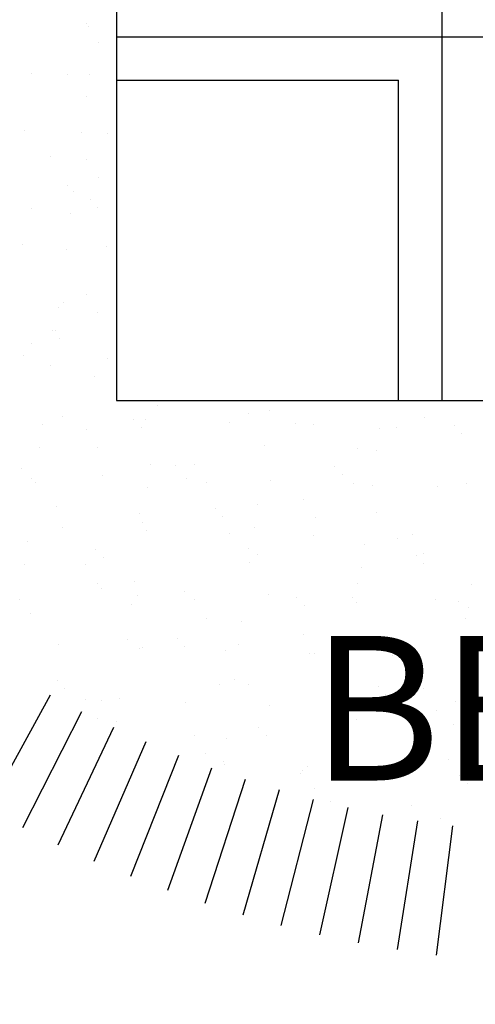
# Model space of a CAD drawing. Units: millimetres. Extents: x -857 to 54106, y -13666 to 13947.
# Tile 32 of 41: x 31622 to 32096, y 8428 to 9453. Entities that reach past the tile are written whole.
import ezdxf

# ---------------------------------------------------------------- set-up
doc = ezdxf.new("R2010")
doc.units = ezdxf.units.MM
for name, color, linetype, lineweight in [('A-ANNO-DIMS', 2, 'Continuous', 18), ('A-AREA-IDEN', 3, 'Continuous', 18), ('A-FURN', 21, 'Continuous', 18)]:
    doc.layers.add(name, color=color, linetype=linetype, lineweight=lineweight)
for name, color, linetype in [('A-FRN', 11, 'Continuous'), ('A-HT', 15, 'Continuous'), ('L-HT', 1, 'Continuous')]:
    doc.layers.add(name, color=color, linetype=linetype)
doc.styles.get("Standard").update_dxf_attribs({"font": 'arial.ttf'})
doc.dimstyles.new('ISO-25', dxfattribs={"dimtxt": 2.5, "dimasz": 2.5, "dimexe": 1.25, "dimexo": 0.625, "dimtad": 1, "dimtxsty": 'Standard', "dimcen": 2.5, "dimadec": 0, "dimazin": 0, "dimtfac": 1, "dimtmove": 0, "dimatfit": 3, "dimfxl": 1, "dimarcsym": 0})

# ---------------------------------------------------------------- blocks, each defined once
blk = doc.blocks.new('*X18')
at = {"color": 0}
for p, q in [((3.0291, 2.2112), (3.0291, 2.2112)), ((2.489, 2.2062), (2.489, 2.2062)), ((2.6199, 2.2078), (2.6199, 2.2078)), ((2.7478, 2.2072), (2.7478, 2.2072)), ((2.8787, 2.2094), (2.8787, 2.2094)), ((2.9625, 2.2024), (2.9625, 2.2024)), ((2.9885, 2.2058), (2.9885, 2.2058)), ((2.4228, 2.1976), (2.4228, 2.1976)), ((2.5785, 2.1978), (2.5785, 2.1978)), ((2.7342, 2.1981), (2.7342, 2.1981)), ((2.8899, 2.1984), (2.8899, 2.1984)), ((2.8946, 2.1935), (2.8946, 2.1935)), ((3.0456, 2.1987), (3.0456, 2.1987)), ((2.8279, 2.1847), (2.8279, 2.1847)), ((2.8539, 2.1881), (2.8539, 2.1881)), ((2.5191, 2.1757), (2.5191, 2.1757)), ((2.6933, 2.167), (2.6933, 2.167)), ((2.7192, 2.174), (2.7192, 2.174)), ((2.7193, 2.1704), (2.7193, 2.1704)), ((2.76, 2.1758), (2.76, 2.1758)), ((2.9222, 2.1695), (2.9222, 2.1695)), ((3.0813, 2.1669), (3.0813, 2.1669)), ((3.1223, 2.1678), (3.1223, 2.1678)), ((2.4246, 2.1567), (2.4246, 2.1567)), ((2.5525, 2.1561), (2.5525, 2.1561)), ((2.6254, 2.158), (2.6254, 2.158)), ((2.6875, 2.161), (2.6875, 2.161)), ((2.7284, 2.1655), (2.7284, 2.1655)), ((2.8184, 2.1626), (2.8184, 2.1626)), ((2.9463, 2.162), (2.9463, 2.162)), ((3.1315, 2.1594), (3.1315, 2.1594)), ((2.5587, 2.1493), (2.5587, 2.1493)), ((2.5847, 2.1527), (2.5847, 2.1527)), ((2.3662, 2.1341), (2.3662, 2.1341)), ((2.3688, 2.1318), (2.3688, 2.1318)), ((2.4501, 2.135), (2.4501, 2.135)), ((2.4908, 2.1403), (2.4908, 2.1403)), ((2.5219, 2.1344), (2.5219, 2.1344)), ((2.6776, 2.1347), (2.6776, 2.1347)), ((2.8333, 2.135), (2.8333, 2.135)), ((2.989, 2.1353), (2.989, 2.1353)), ((3.1447, 2.1356), (3.1447, 2.1356)), ((2.3872, 2.1207), (2.3872, 2.1207)), ((2.4241, 2.1315), (2.4241, 2.1315)), ((2.5429, 2.121), (2.5429, 2.121)), ((2.5689, 2.1301), (2.5689, 2.1301)), ((2.5781, 2.1216), (2.5781, 2.1216)), ((2.6987, 2.1213), (2.6987, 2.1213)), ((2.7719, 2.1257), (2.7719, 2.1257)), ((2.8544, 2.1216), (2.8544, 2.1216)), ((2.972, 2.1239), (2.972, 2.1239)), ((3.0101, 2.1218), (3.0101, 2.1218)), ((3.1658, 2.1221), (3.1658, 2.1221)), ((2.4922, 2.1098), (2.4922, 2.1098)), ((2.623, 2.1115), (2.623, 2.1115)), ((2.751, 2.1109), (2.751, 2.1109)), ((2.886, 2.1157), (2.886, 2.1157)), ((2.9812, 2.1155), (2.9812, 2.1155)), ((3.0169, 2.1174), (3.0169, 2.1174)), ((3.1448, 2.1168), (3.1448, 2.1168)), ((3.1692, 2.1002), (3.1692, 2.1002)), ((3.0752, 2.0878), (3.0752, 2.0878)), ((3.1432, 2.0968), (3.1432, 2.0968)), ((2.8216, 2.08), (2.8216, 2.08)), ((3.0086, 2.079), (3.0086, 2.079)), ((3.0247, 2.0756), (3.0247, 2.0756)), ((3.0346, 2.0825), (3.0346, 2.0825)), ((2.8215, 2.0663), (2.8215, 2.0663)), ((2.8309, 2.0716), (2.8309, 2.0716)), ((2.9, 2.0647), (2.9, 2.0647)), ((2.9303, 2.0732), (2.9303, 2.0732)), ((2.9407, 2.0701), (2.9407, 2.0701)), ((2.9494, 2.0657), (2.9494, 2.0657)), ((3.0845, 2.0705), (3.0845, 2.0705)), ((3.086, 2.0735), (3.086, 2.0735)), ((2.874, 2.0613), (2.874, 2.0613)), ((2.8061, 2.0524), (2.8061, 2.0524)), ((2.8744, 2.0317), (2.8744, 2.0317)), ((3.0744, 2.03), (3.0744, 2.03)), ((2.8891, 2.0194), (2.8891, 2.0194)), ((3.02, 2.0211), (3.02, 2.0211)), ((3.0837, 2.0216), (3.0837, 2.0216)), ((3.1479, 2.0205), (3.1479, 2.0205)), ((2.8737, 2.0098), (2.8737, 2.0098)), ((3.0294, 2.0101), (3.0294, 2.0101)), ((3.1851, 2.0104), (3.1851, 2.0104)), ((2.8947, 1.9964), (2.8947, 1.9964)), ((3.0505, 1.9966), (3.0505, 1.9966)), ((3.2062, 1.9969), (3.2062, 1.9969)), ((2.9241, 1.9861), (2.9241, 1.9861)), ((2.9333, 1.9777), (2.9333, 1.9777)), ((3.0876, 1.9742), (3.0876, 1.9742)), ((3.1272, 1.9817), (3.1272, 1.9817)), ((3.1893, 1.9734), (3.1893, 1.9734)), ((3.2153, 1.9768), (3.2153, 1.9768)), ((3.2185, 1.9759), (3.2185, 1.9759)), ((2.8247, 1.9699), (2.8247, 1.9699)), ((2.9526, 1.9693), (2.9526, 1.9693)), ((3.1213, 1.9644), (3.1213, 1.9644)), ((3.0547, 1.9556), (3.0547, 1.9556)), ((3.0807, 1.9591), (3.0807, 1.9591)), ((2.8149, 1.9477), (2.8149, 1.9477)), ((2.9461, 1.9414), (2.9461, 1.9414)), ((2.9707, 1.948), (2.9707, 1.948)), ((2.9868, 1.9467), (2.9868, 1.9467)), ((3.1264, 1.9483), (3.1264, 1.9483)), ((2.8522, 1.929), (2.8522, 1.929)), ((2.9201, 1.9379), (2.9201, 1.9379)), ((2.9768, 1.9378), (2.9768, 1.9378)), ((3.1769, 1.9361), (3.1769, 1.9361)), ((2.8115, 1.9236), (2.8115, 1.9236)), ((2.8923, 1.9231), (2.8923, 1.9231)), ((3.0232, 1.9247), (3.0232, 1.9247)), ((3.1511, 1.9241), (3.1511, 1.9241)), ((3.1861, 1.9277), (3.1861, 1.9277)), ((2.8265, 1.894), (2.8265, 1.894)), ((2.914, 1.8846), (2.914, 1.8846)), ((3.0266, 1.8922), (3.0266, 1.8922)), ((3.0358, 1.8838), (3.0358, 1.8838)), ((3.0697, 1.8849), (3.0697, 1.8849)), ((3.2255, 1.8852), (3.2255, 1.8852)), ((3.2296, 1.8878), (3.2296, 1.8878)), ((2.8278, 1.8736), (2.8278, 1.8736)), ((2.9351, 1.8712), (2.9351, 1.8712)), ((2.9557, 1.873), (2.9557, 1.873)), ((3.0908, 1.8779), (3.0908, 1.8779)), ((3.0908, 1.8714), (3.0908, 1.8714)), ((3.2217, 1.8795), (3.2217, 1.8795)), ((3.2465, 1.8717), (3.2465, 1.8717)), ((2.8763, 1.8484), (2.8763, 1.8484)), ((3.2354, 1.85), (3.2354, 1.85)), ((3.2614, 1.8534), (3.2614, 1.8534)), ((2.8855, 1.8399), (2.8855, 1.8399)), ((3.0793, 1.8439), (3.0793, 1.8439)), ((3.1674, 1.841), (3.1674, 1.841)), ((2.8954, 1.8267), (2.8954, 1.8267)), ((3.0263, 1.8284), (3.0263, 1.8284)), ((3.1008, 1.8323), (3.1008, 1.8323)), ((3.1268, 1.8357), (3.1268, 1.8357)), ((3.1542, 1.8278), (3.1542, 1.8278)), ((2.8553, 1.8225), (2.8553, 1.8225)), ((2.9662, 1.8145), (2.9662, 1.8145)), ((2.9922, 1.818), (2.9922, 1.818)), ((3.011, 1.8228), (3.011, 1.8228)), ((3.0329, 1.8233), (3.0329, 1.8233)), ((3.1667, 1.8231), (3.1667, 1.8231)), ((2.8983, 1.8056), (2.8983, 1.8056)), ((2.8316, 1.7968), (2.8316, 1.7968)), ((2.8576, 1.8002), (2.8576, 1.8002)), ((2.929, 1.8), (2.929, 1.8)), ((3.1291, 1.7983), (3.1291, 1.7983)), ((3.0939, 1.7815), (3.0939, 1.7815)), ((3.1383, 1.7899), (3.1383, 1.7899)), ((3.2248, 1.7832), (3.2248, 1.7832)), ((2.831, 1.7773), (2.831, 1.7773)), ((2.9589, 1.7766), (2.9589, 1.7766)), ((2.9544, 1.7594), (2.9544, 1.7594)), ((3.1101, 1.7597), (3.1101, 1.7597)), ((3.2658, 1.7599), (3.2658, 1.7599)), ((2.9788, 1.7544), (2.9788, 1.7544)), ((3.1818, 1.75), (3.1818, 1.75)), ((2.8198, 1.7457), (2.8198, 1.7457)), ((2.9755, 1.7459), (2.9755, 1.7459)), ((2.988, 1.746), (2.988, 1.746)), ((3.1312, 1.7462), (3.1312, 1.7462)), ((2.8986, 1.7304), (2.8986, 1.7304)), ((3.0295, 1.7321), (3.0295, 1.7321)), ((3.1574, 1.7314), (3.1574, 1.7314)), ((3.2815, 1.7266), (3.2815, 1.7266)), ((3.1729, 1.7123), (3.1729, 1.7123)), ((3.2135, 1.7176), (3.2135, 1.7176)), ((2.8285, 1.7106), (2.8285, 1.7106)), ((2.8377, 1.7021), (2.8377, 1.7021)), ((3.0315, 1.7061), (3.0315, 1.7061)), ((3.1469, 1.7089), (3.1469, 1.7089)), ((3.2316, 1.7044), (3.2316, 1.7044)), ((2.8957, 1.6973), (2.8957, 1.6973)), ((3.0123, 1.6911), (3.0123, 1.6911)), ((3.0383, 1.6946), (3.0383, 1.6946)), ((3.0514, 1.6976), (3.0514, 1.6976)), ((3.079, 1.6999), (3.079, 1.6999)), ((3.2071, 1.6979), (3.2071, 1.6979)), ((3.2408, 1.696), (3.2408, 1.696)), ((3.228, 1.6868), (3.228, 1.6868))]:
    blk.add_line(p, q, dxfattribs=at)
blk = doc.blocks.new('A$C6796526C')
at = {"layer": 'A-FRN'}
blk.add_lwpolyline([(0.65, 2.8), (0.65, 0.9), (2.25, 0.9), (2.25, 2.8)], dxfattribs=at)
at = {"layer": 'A-HT'}
for p, q in [((2.7397, 1.2871), (2.8886, 1.2683)), ((2.734, 1.2466), (2.8821, 1.2232)), ((2.727, 1.2064), (2.8743, 1.1783)), ((2.7187, 1.1664), (2.8651, 1.1337)), ((2.7092, 1.1267), (2.8544, 1.0894)), ((2.6984, 1.0873), (2.8424, 1.0455)), ((2.6864, 1.0483), (2.829, 1.0019)), ((2.6731, 1.0096), (2.8143, 0.9588)), ((2.6587, 0.9714), (2.7982, 0.9162)), ((2.6431, 0.9337), (2.7807, 0.8741)), ((2.6263, 0.8965), (2.762, 0.8326)), ((2.6083, 0.8598), (2.742, 0.7917)), ((2.5892, 0.8237), (2.7206, 0.7515))]:
    blk.add_line(p, q, dxfattribs=at)
at = {"layer": 'L-HT'}
for p, q in [((1.8309, 0.9), (1.8309, 2.2094)), ((0.65, 1.2749), (2.25, 1.2749)), ((1.8809, 0.9), (1.8809, 1.2249)), ((2.25, 1.2249), (1.8809, 1.2249))]:
    blk.add_line(p, q, dxfattribs=at)
at = {"layer": 'A-HT', "extrusion": (0, 0, -1), "zscale": -1, "rotation": 180}
blk.add_blockref('*X18', (0.55, 3), dxfattribs=at)
blk = doc.blocks.new('*D47')
at = {"layer": 'A-ANNO-DIMS', "color": 0, "lineweight": -2, "transparency": 16777216}
for p, q in [((30909.3, 8468.4), (30909.3, 8061.1)), ((33620.1, 8468.4), (33620.1, 8061.1)), ((30911.8, 8062.4), (33617.6, 8062.4))]:
    blk.add_line(p, q, dxfattribs=at)
at = {"layer": 'A-ANNO-DIMS', "color": 0, "transparency": 16777216}
for points in [[(30911.8, 8062.8), (30911.8, 8062), (30909.3, 8062.4)], [(33617.6, 8062.8), (33617.6, 8062), (33620.1, 8062.4)]]:
    blk.add_solid(points, dxfattribs=at)
at = {"layer": 'Defpoints', "color": 0, "transparency": 16777216}
for p in [(30909.3, 8469), (33620.1, 8469), (33620.1, 8062.4)]:
    blk.add_point(p, dxfattribs=at)
at = {"layer": 'A-ANNO-DIMS', "color": 0, "transparency": 16777216, "insert": (32264.7, 8064.3), "char_height": 2.5, "attachment_point": 5}
blk.add_mtext('ROUND BED 2711 TYP.', dxfattribs=at)

msp = doc.modelspace()

# ---------------------------------------------------------------- block references
at = {"layer": 'A-FURN', "xscale": 903.6084929786902, "yscale": 903.6084929786902, "zscale": 903.6084929786902, "rotation": 269.9999999999988}
msp.add_blockref('A$C6796526C', (30909.253, 11089.463), dxfattribs=at)

# ---------------------------------------------------------------- texts
at = {"layer": 'A-AREA-IDEN', "insert": (31924.893, 8811.521), "char_height": 150.48461, "attachment_point": 1}
msp.add_mtext_dynamic_manual_height_columns('\\pxt0;BEDROOM 2', width=2554.22693, gutter_width=18810.576, heights=[2595.835], dxfattribs=at)

# ---------------------------------------------------------------- dimensions: what is measured, and where the dimension line sits
at = {"layer": 'A-ANNO-DIMS'}
dim = msp.add_linear_dim(base=(33620.079, 8062.375), p1=(30909.254, 8468.999), p2=(33620.079, 8468.999), text='ROUND BED <> TYP.', dimstyle='ISO-25', override={"dimdec": 0, "dimrnd": 0, "dimzin": 0, "dimlunit": 2}, dxfattribs=at)
dim.commit()
dim.dimension.update_dxf_attribs({"geometry": '*D47', "text_midpoint": (32264.666, 8064.293)})

doc.saveas('drawing.dxf')
